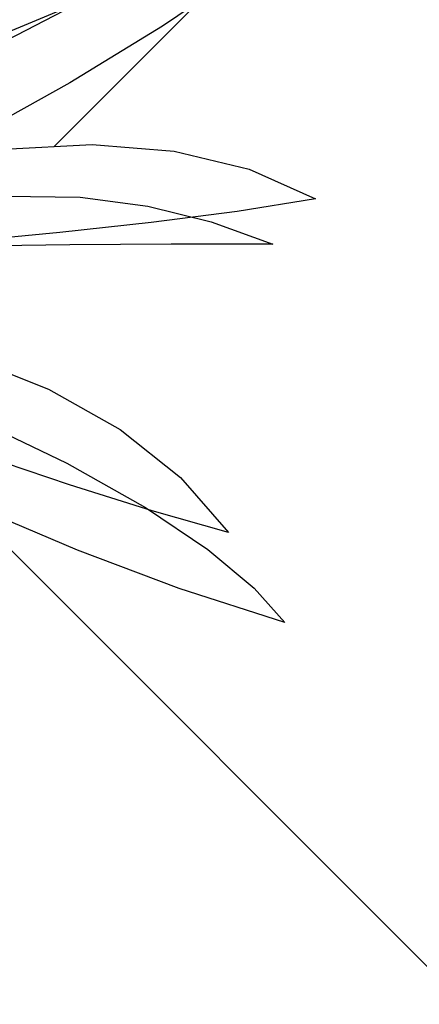
# Model space of a CAD drawing. Units: inches. Extents: x 3590 to 5167, y 65 to 1917.
# Tile 32 of 100: x 4960.64 to 4967.82, y 1339.27 to 1356.94. Entities that reach past the tile are written whole.
import ezdxf

# ---------------------------------------------------------------- set-up
doc = ezdxf.new("R2010")
doc.units = ezdxf.units.IN
doc.layers.add('A-FLOR-PATT', color=8, linetype='Continuous', lineweight=13)
doc.layers.add('L-PLNT', color=94, linetype='Continuous', lineweight=18)
doc.layers.add('DIENHOA', color=3, linetype='Continuous')

# ---------------------------------------------------------------- blocks, each defined once
blk = doc.blocks.new('Cay03_mb')
at = {"layer": 'DIENHOA'}
for p, q in [((363.69, 192.89), (290.19, 154.87)), ((314.63, 54.14), (369.18, 53.28)), ((369.18, 53.28), (418.6, 46.82)), ((418.6, 46.82), (464.87, 35.24)), ((464.87, 35.24), (510, 19)), ((361.61, 18.5), (289.03, 17.44)), ((435.8, 18.92), (361.61, 18.5)), ((510, 19), (435.8, 18.92)), ((289.55, -107.64), (359.29, -141.1)), ((359.29, -141.1), (416.89, -173.51)), ((367.1, -204.83), (296, -174.69)), ((416.89, -173.51), (462.55, -204.2)), ((441.55, -232.67), (367.1, -204.83)), ((462.55, -204.2), (496.5, -232.48)), ((518.93, -257.68), (441.55, -232.67)), ((496.5, -232.48), (518.93, -257.68))]:
    blk.add_line(p, q, dxfattribs=at)
for points in [[(496.74, 224.01), (429.38, 178.44), (361.6, 136.93), (294.07, 99.46), (227.46, 66.07), (162.44, 36.74), (99.68, 11.49), (39.84, -9.67), (-16.39, -26.73)], [(-16.39, -26.73), (75.38, 37.88), (160.06, 91.82), (237.27, 135.67), (306.57, 170.01), (367.58, 195.44), (419.88, 212.52), (463.07, 221.85), (496.74, 224.01)], [(23.69, -5.44), (99.27, 29.67), (173.22, 57.09), (244.79, 76.69), (313.26, 88.31), (377.88, 91.81), (437.93, 87.02), (492.67, 73.8), (541.37, 52)], [(541.37, 52), (484.11, 42.89), (421.18, 34.83), (354.36, 27.58), (285.41, 20.89), (216.1, 14.49), (148.2, 8.14), (83.47, 1.58), (23.69, -5.44)], [(-16.39, -26.73), (66.95, -26.58), (145.58, -32.71), (218.77, -44.94), (285.79, -63.12), (345.92, -87.06), (398.42, -116.6), (442.57, -151.57), (477.63, -191.79)], [(477.63, -191.79), (421.82, -176.03), (361.32, -156.94), (297.62, -135.49), (232.22, -112.64), (166.63, -89.37), (102.33, -66.65), (40.82, -45.45), (-16.39, -26.73)]]:
    blk.add_lwpolyline(points, dxfattribs=at)

msp = doc.modelspace()

# ---------------------------------------------------------------- hatches: boundary and pattern name
at = {"layer": 'A-FLOR-PATT', "transparency": 33554687}
h = msp.add_hatch(dxfattribs=at)
h.set_pattern_fill('AR-HBONE', color=256, scale=0.2)
h.set_pattern_definition([(45, (-588.972, 0), (0, 28.73682), [60.96, -20.32]), (135, (-574.604, 14.368), (3e-15, 28.73682), [60.96, -20.32])])
h.paths.add_polyline_path([(5071.274, 1796.999), (4933.274, 1796.999), (4933.274, 1753.999), (4962.774, 1753.999, -0.414214), (4928.774, 1719.999), (4933.274, 1718.999), (4933.274, 1334.999), (5071.274, 1334.999)])
h.paths.add_polyline_path([(4951.78, 1521.077), (4951.715, 1521.04), (4951.563, 1520.895)], flags=16)
h.paths.add_polyline_path([(4952.267, 1521.376), (4952.198, 1521.371), (4952.198, 1521.356)], flags=0)
h.paths.add_polyline_path([(4967.051, 1529.728), (4965.231, 1528.694), (4963.411, 1527.714), (4961.756, 1526.851), (4963.589, 1527.449), (4964.036, 1527.478), (4962.975, 1527.249), (4961.76, 1526.852), (4959.792, 1525.834), (4958.005, 1524.895), (4956.24, 1523.93), (4954.504, 1522.919), (4954.129, 1522.682), (4953.361, 1521.997), (4953.366, 1521.998), (4953.605, 1522.064), (4955.106, 1522.761), (4956.921, 1523.434), (4958.678, 1523.915), (4960.358, 1524.2), (4961.945, 1524.286), (4964.171, 1524.108), (4965.958, 1523.309), (4963.863, 1522.976), (4965.187, 1522.499), (4963.366, 1522.497), (4961.545, 1522.487), (4959.764, 1522.461), (4958.304, 1522.419), (4957.974, 1522.388), (4956.307, 1522.232), (4954.718, 1522.071), (4953.251, 1521.899), (4953.525, 1521.623), (4954.331, 1521.379), (4956.243, 1521.23), (4958.039, 1520.93), (4959.684, 1520.483), (4961.16, 1519.896), (4963.107, 1518.8), (4964.393, 1517.325), (4962.973, 1517.726), (4964.558, 1516.661), (4965.407, 1515.708), (4963.507, 1516.322), (4961.68, 1517.005), (4959.935, 1517.745), (4958.282, 1518.528), (4956.732, 1519.343), (4955.295, 1520.175), (4954.672, 1520.572), (4954.513, 1520.627), (4955.658, 1519.318), (4956.703, 1517.982), (4957.644, 1516.647), (4958.485, 1515.334), (4959.55, 1513.524), (4960.438, 1511.769), (4958.841, 1513.62), (4957.452, 1515.325), (4955.819, 1517.459), (4956.665, 1515.448), (4957.111, 1513.923), (4957.447, 1511.714), (4957.076, 1509.793), (4956.538, 1511.11), (4955.992, 1512.569), (4955.444, 1514.125), (4954.898, 1515.735), (4954.357, 1517.356), (4953.824, 1518.943), (4953.305, 1520.452), (4953.065, 1521.116), (4952.971, 1521.146), (4952.949, 1521.086), (4952.73, 1520.199), (4953.37, 1518.024), (4953.757, 1516.373), (4954.051, 1514.765), (4954.264, 1513.221), (4954.471, 1511.131), (4954.497, 1510.402), (4954.409, 1511.76), (4954.264, 1513.221), (4954.051, 1514.765), (4953.757, 1516.373), (4953.37, 1518.024), (4952.877, 1519.698), (4952.716, 1520.141), (4952.533, 1519.059), (4952.374, 1517.789), (4952.219, 1516.312), (4952.046, 1514.6), (4951.833, 1512.626), (4951.557, 1510.363), (4951.203, 1512.168), (4950.852, 1514.339), (4950.985, 1516.376), (4951.66, 1518.286), (4952.593, 1520.481), (4952.357, 1521.13), (4951.855, 1520.328), (4950.839, 1518.908), (4949.777, 1517.587), (4948.916, 1516.617), (4948.111, 1515.256), (4947.089, 1513.554), (4945.889, 1511.615), (4946.326, 1513.402), (4946.562, 1514.249), (4945.528, 1513.327), (4944.581, 1512.531), (4946.018, 1514.508), (4947.204, 1516.048), (4947.893, 1517.313), (4949.307, 1518.764), (4950.414, 1519.767), (4950.451, 1519.806), (4952.267, 1521.376), (4951.645, 1521.493), (4950.404, 1521.18), (4948.044, 1520.359), (4946.119, 1519.452), (4944.572, 1518.475), (4943.35, 1517.443), (4941.997, 1515.92), (4941.661, 1515.275), (4942.813, 1516.99), (4944.572, 1518.475), (4946.119, 1519.452), (4948.044, 1520.359), (4950.404, 1521.18), (4951.645, 1521.493), (4949.647, 1521.868), (4948.6, 1521.756), (4947.126, 1521.57), (4945.42, 1521.348), (4943.45, 1521.105), (4941.183, 1520.856), (4942.86, 1521.613), (4943.873, 1522.03), (4942.952, 1521.909), (4941.41, 1521.485), (4939.543, 1520.67), (4938.968, 1520.226), (4940.733, 1521.299), (4942.952, 1521.909), (4943.702, 1522.008), (4945.894, 1522.7), (4947.565, 1522.714), (4948.921, 1522.566), (4951.131, 1522.183), (4950.971, 1522.297), (4948.129, 1523.006), (4946.035, 1523.707), (4944.232, 1524.521), (4942.707, 1525.461), (4941.444, 1526.537), (4940.43, 1527.761), (4939.649, 1529.143), (4941.421, 1528.122), (4943.147, 1527.132), (4944.841, 1526.175), (4946.514, 1525.25), (4948.179, 1524.359), (4948.365, 1524.263), (4946.475, 1526.045), (4945.181, 1527.54), (4944.19, 1529.033), (4943.496, 1530.54), (4943.278, 1531.36), (4942.498, 1531.919), (4943.114, 1531.762), (4942.959, 1533.659), (4944.14, 1531.989), (4944.612, 1531.323), (4946.202, 1530.463), (4947.486, 1529.509), (4948.79, 1528.226), (4950.368, 1526.237), (4949.485, 1528.155), (4948.851, 1530.123), (4948.491, 1532.041), (4948.381, 1533.918), (4948.501, 1535.76), (4948.827, 1537.573), (4949.418, 1535.565), (4949.957, 1533.569), (4950.464, 1531.586), (4950.961, 1529.617), (4951.391, 1527.954), (4951.724, 1530.687), (4952.201, 1532.58), (4952.889, 1534.33), (4953.77, 1535.951), (4954.827, 1537.46), (4954.521, 1535.39), (4954.273, 1533.937), (4955.58, 1535.663), (4956.748, 1536.739), (4956.159, 1534.78), (4955.589, 1532.873), (4955.043, 1531.006), (4954.525, 1529.166), (4954.038, 1527.341), (4953.638, 1525.733), (4953.611, 1525.586), (4953.398, 1524.166), (4953.382, 1524.009), (4954.07, 1525.476), (4954.912, 1527.022), (4956.136, 1528.894), (4957.847, 1530.577), (4959.376, 1531.54), (4958.256, 1530.104), (4957.143, 1528.663), (4956.066, 1527.243), (4955.056, 1525.871), (4954.141, 1524.571), (4953.352, 1523.372), (4953.311, 1523.303), (4953.273, 1522.925), (4953.261, 1522.382), (4954.103, 1523.373), (4954.63, 1524.284), (4955.961, 1526.358), (4957.23, 1528.13), (4958.421, 1529.609), (4960.037, 1531.368), (4961.374, 1532.375), (4962.101, 1532.77), (4961.07, 1531.061), (4959.987, 1529.438), (4958.869, 1527.908), (4958.15, 1527.007), (4959.803, 1528.003), (4961.589, 1528.793), (4963.391, 1529.328), (4965.211, 1529.632)], flags=16)
h.paths.add_polyline_path([(4962.944, 1523.182), (4961.107, 1523.422), (4960.392, 1523.362), (4962.35, 1523.331)], flags=0)
h.paths.add_polyline_path([(5049.541, 1584.551), (5049.476, 1584.515), (5049.325, 1584.37)], flags=16)
h.paths.add_polyline_path([(5050.028, 1584.851), (5049.959, 1584.845), (5049.959, 1584.83)], flags=0)
h.paths.add_polyline_path([(5042.333, 1581.949), (5043.88, 1582.926), (5045.806, 1583.833), (5048.165, 1584.654), (5049.406, 1584.967), (5047.408, 1585.342), (5046.361, 1585.231), (5044.888, 1585.044), (5043.181, 1584.822), (5041.211, 1584.579), (5038.944, 1584.33), (5040.622, 1585.087), (5041.634, 1585.504), (5040.713, 1585.383), (5039.171, 1584.959), (5037.304, 1584.144), (5036.729, 1583.7), (5038.494, 1584.773), (5040.713, 1585.383), (5041.463, 1585.482), (5043.655, 1586.174), (5045.326, 1586.188), (5046.682, 1586.04), (5048.893, 1585.657), (5048.732, 1585.771), (5045.891, 1586.48), (5043.796, 1587.181), (5041.994, 1587.996), (5040.468, 1588.935), (5039.205, 1590.011), (5038.191, 1591.235), (5037.41, 1592.617), (5039.182, 1591.596), (5040.909, 1590.607), (5042.602, 1589.649), (5044.275, 1588.724), (5045.94, 1587.833), (5046.126, 1587.738), (5044.237, 1589.519), (5042.942, 1591.015), (5041.952, 1592.508), (5041.257, 1594.014), (5041.039, 1594.834), (5040.26, 1595.393), (5040.875, 1595.237), (5040.721, 1597.133), (5041.901, 1595.463), (5042.373, 1594.798), (5043.963, 1593.938), (5045.247, 1592.983), (5046.552, 1591.701), (5048.129, 1589.712), (5047.247, 1591.63), (5046.613, 1593.597), (5046.252, 1595.515), (5046.142, 1597.392), (5046.262, 1599.234), (5046.588, 1601.047), (5047.179, 1599.039), (5047.718, 1597.043), (5048.225, 1595.06), (5048.722, 1593.091), (5049.152, 1591.429), (5049.485, 1594.161), (5049.962, 1596.054), (5050.65, 1597.804), (5051.532, 1599.425), (5052.589, 1600.934), (5052.283, 1598.864), (5052.034, 1597.411), (5053.341, 1599.137), (5054.509, 1600.213), (5053.92, 1598.254), (5053.35, 1596.348), (5052.805, 1594.48), (5052.286, 1592.64), (5051.799, 1590.815), (5051.4, 1589.207), (5051.373, 1589.06), (5051.159, 1587.64), (5051.143, 1587.483), (5051.831, 1588.95), (5052.673, 1590.496), (5053.898, 1592.368), (5055.608, 1594.051), (5057.137, 1595.014), (5056.017, 1593.578), (5054.904, 1592.137), (5053.828, 1590.717), (5052.817, 1589.345), (5051.902, 1588.046), (5051.113, 1586.846), (5051.072, 1586.777), (5051.034, 1586.399), (5051.022, 1585.856), (5051.864, 1586.847), (5052.391, 1587.758), (5053.723, 1589.832), (5054.991, 1591.604), (5056.182, 1593.083), (5057.798, 1594.842), (5059.135, 1595.849), (5059.863, 1596.244), (5058.831, 1594.535), (5057.749, 1592.912), (5056.63, 1591.382), (5055.912, 1590.482), (5057.564, 1591.477), (5059.35, 1592.267), (5061.152, 1592.802), (5062.972, 1593.106), (5064.812, 1593.203), (5062.992, 1592.169), (5061.172, 1591.188), (5059.518, 1590.325), (5061.35, 1590.924), (5061.797, 1590.952), (5060.737, 1590.723), (5059.521, 1590.326), (5057.553, 1589.308), (5055.766, 1588.369), (5054.002, 1587.404), (5052.265, 1586.393), (5051.891, 1586.156), (5051.122, 1585.471), (5051.127, 1585.472), (5051.366, 1585.538), (5052.867, 1586.235), (5054.682, 1586.908), (5056.439, 1587.389), (5058.12, 1587.675), (5059.706, 1587.76), (5061.933, 1587.583), (5063.719, 1586.783), (5061.624, 1586.45), (5062.949, 1585.973), (5061.127, 1585.971), (5059.307, 1585.961), (5057.525, 1585.935), (5056.065, 1585.893), (5055.735, 1585.862), (5054.068, 1585.707), (5052.479, 1585.546), (5051.012, 1585.373), (5051.286, 1585.097), (5052.092, 1584.853), (5054.004, 1584.704), (5055.8, 1584.404), (5057.446, 1583.958), (5058.921, 1583.37), (5060.868, 1582.274), (5062.154, 1580.799), (5060.734, 1581.2), (5062.32, 1580.135), (5063.168, 1579.182), (5061.269, 1579.796), (5059.441, 1580.479), (5057.696, 1581.219), (5056.043, 1582.003), (5054.493, 1582.817), (5053.057, 1583.649), (5052.433, 1584.047), (5052.274, 1584.101), (5053.42, 1582.793), (5054.464, 1581.457), (5055.405, 1580.121), (5056.247, 1578.809), (5057.311, 1576.998), (5058.199, 1575.244), (5056.602, 1577.094), (5055.213, 1578.799), (5053.58, 1580.933), (5054.427, 1578.922), (5054.872, 1577.397), (5055.208, 1575.189), (5054.838, 1573.267), (5054.299, 1574.584), (5053.754, 1576.043), (5053.206, 1577.599), (5052.659, 1579.209), (5052.118, 1580.83), (5051.585, 1582.417), (5051.066, 1583.927), (5050.826, 1584.59), (5050.733, 1584.62), (5050.711, 1584.561), (5050.491, 1583.673), (5051.131, 1581.498), (5051.518, 1579.847), (5051.813, 1578.24), (5052.026, 1576.695), (5052.233, 1574.605), (5052.258, 1573.876), (5052.17, 1575.234), (5052.026, 1576.695), (5051.813, 1578.24), (5051.518, 1579.847), (5051.131, 1581.498), (5050.638, 1583.172), (5050.477, 1583.615), (5050.294, 1582.533), (5050.136, 1581.263), (5049.981, 1579.786), (5049.807, 1578.074), (5049.594, 1576.1), (5049.318, 1573.837), (5048.965, 1575.642), (5048.613, 1577.813), (5048.747, 1579.85), (5049.421, 1581.76), (5050.354, 1583.955), (5050.118, 1584.604), (5049.616, 1583.802), (5048.6, 1582.382), (5047.538, 1581.061), (5046.677, 1580.091), (5045.872, 1578.73), (5044.85, 1577.028), (5043.651, 1575.089), (5044.087, 1576.877), (5044.324, 1577.723), (5043.289, 1576.801), (5042.342, 1576.005), (5043.779, 1577.982), (5044.966, 1579.522), (5045.655, 1580.787), (5047.068, 1582.239), (5048.175, 1583.241), (5048.213, 1583.28), (5050.028, 1584.851), (5049.406, 1584.967), (5048.165, 1584.654), (5045.806, 1583.833), (5043.88, 1582.926), (5042.333, 1581.949), (5041.111, 1580.917), (5039.758, 1579.394), (5039.423, 1578.749), (5040.575, 1580.464)], flags=16)
h.paths.add_polyline_path([(4954.799, 1533.12), (4954.262, 1532.079), (4953.831, 1530.935), (4953.505, 1529.636), (4953.283, 1528.133), (4953.167, 1526.376), (4953.156, 1524.315), (4953.277, 1521.236), (4952.802, 1521.842), (4951.557, 1521.998), (4950.976, 1521.961), (4952.661, 1521.941), (4952.802, 1521.842), (4953.152, 1523.593), (4953.167, 1526.376), (4953.283, 1528.133), (4953.609, 1530.346), (4954.456, 1532.592)], flags=0)
h.paths.add_polyline_path([(5050.563, 1585.316), (5049.318, 1585.472), (5048.737, 1585.435), (5050.422, 1585.415), (5050.563, 1585.316), (5050.914, 1587.067), (5050.928, 1589.851), (5051.045, 1591.607), (5051.371, 1593.82), (5052.217, 1596.066), (5052.56, 1596.594), (5052.024, 1595.554), (5051.592, 1594.409), (5051.266, 1593.11), (5051.045, 1591.607), (5050.928, 1589.851), (5050.918, 1587.789), (5051.038, 1584.71)], flags=0)
h.paths.add_polyline_path([(5058.153, 1586.836), (5060.111, 1586.805), (5060.705, 1586.656), (5058.868, 1586.896)], flags=0)
h.paths.add_polyline_path([(5049.541, 1430.936), (5049.476, 1430.9), (5049.325, 1430.755)], flags=16)
h.paths.add_polyline_path([(5050.028, 1431.236), (5049.959, 1431.231), (5049.959, 1431.215)], flags=0)
h.paths.add_polyline_path([(5046.588, 1447.432), (5047.179, 1445.425), (5047.718, 1443.429), (5048.225, 1441.446), (5048.722, 1439.476), (5049.152, 1437.814), (5049.485, 1440.546), (5049.962, 1442.439), (5050.65, 1444.189), (5051.532, 1445.811), (5052.589, 1447.319), (5052.283, 1445.249), (5052.034, 1443.796), (5053.341, 1445.522), (5054.509, 1446.598), (5053.92, 1444.64), (5053.35, 1442.733), (5052.805, 1440.865), (5052.286, 1439.025), (5051.799, 1437.201), (5051.4, 1435.592), (5051.373, 1435.445), (5051.159, 1434.025), (5051.143, 1433.868), (5051.831, 1435.335), (5052.673, 1436.881), (5053.898, 1438.753), (5055.608, 1440.436), (5057.137, 1441.4), (5056.017, 1439.963), (5054.904, 1438.522), (5053.828, 1437.102), (5052.817, 1435.73), (5051.902, 1434.431), (5051.113, 1433.231), (5051.072, 1433.162), (5051.034, 1432.784), (5051.022, 1432.242), (5051.864, 1433.232), (5052.391, 1434.143), (5053.723, 1436.217), (5054.991, 1437.989), (5056.182, 1439.468), (5057.798, 1441.227), (5059.135, 1442.235), (5059.863, 1442.629), (5058.831, 1440.921), (5057.749, 1439.298), (5056.63, 1437.767), (5055.912, 1436.867), (5057.564, 1437.863), (5059.35, 1438.652), (5061.152, 1439.187), (5062.972, 1439.491), (5064.812, 1439.588), (5062.992, 1438.554), (5061.172, 1437.573), (5059.518, 1436.71), (5061.35, 1437.309), (5061.797, 1437.337), (5060.737, 1437.108), (5059.521, 1436.711), (5057.553, 1435.693), (5055.766, 1434.754), (5054.002, 1433.789), (5052.265, 1432.778), (5051.891, 1432.541), (5051.122, 1431.856), (5051.127, 1431.857), (5051.366, 1431.923), (5052.867, 1432.62), (5054.682, 1433.293), (5056.439, 1433.775), (5058.12, 1434.06), (5059.706, 1434.145), (5061.933, 1433.968), (5063.719, 1433.168), (5061.624, 1432.835), (5062.949, 1432.358), (5061.127, 1432.357), (5059.307, 1432.346), (5057.525, 1432.32), (5056.065, 1432.278), (5055.735, 1432.248), (5054.068, 1432.092), (5052.479, 1431.931), (5051.012, 1431.759), (5051.286, 1431.482), (5052.092, 1431.238), (5054.004, 1431.089), (5055.8, 1430.789), (5057.446, 1430.343), (5058.921, 1429.755), (5060.868, 1428.66), (5062.154, 1427.185), (5060.734, 1427.585), (5062.32, 1426.52), (5063.168, 1425.567), (5061.269, 1426.181), (5059.441, 1426.865), (5057.696, 1427.604), (5056.043, 1428.388), (5054.493, 1429.202), (5053.057, 1430.034), (5052.433, 1430.432), (5052.274, 1430.487), (5053.42, 1429.178), (5054.464, 1427.842), (5055.405, 1426.506), (5056.247, 1425.194), (5057.311, 1423.383), (5058.199, 1421.629), (5056.602, 1423.479), (5055.213, 1425.184), (5053.58, 1427.318), (5054.427, 1425.307), (5054.872, 1423.782), (5055.208, 1421.574), (5054.838, 1419.652), (5054.299, 1420.97), (5053.754, 1422.428), (5053.206, 1423.984), (5052.659, 1425.595), (5052.118, 1427.215), (5051.585, 1428.802), (5051.066, 1430.312), (5050.826, 1430.975), (5050.733, 1431.005), (5050.711, 1430.946), (5050.491, 1430.058), (5051.131, 1427.883), (5051.518, 1426.232), (5051.813, 1424.625), (5052.026, 1423.081), (5052.233, 1420.991), (5052.258, 1420.261), (5052.17, 1421.619), (5052.026, 1423.081), (5051.813, 1424.625), (5051.518, 1426.232), (5051.131, 1427.883), (5050.638, 1429.558), (5050.477, 1430.001), (5050.294, 1428.918), (5050.136, 1427.648), (5049.981, 1426.171), (5049.807, 1424.459), (5049.594, 1422.485), (5049.318, 1420.222), (5048.965, 1422.028), (5048.613, 1424.199), (5048.747, 1426.235), (5049.421, 1428.146), (5050.354, 1430.34), (5050.118, 1430.989), (5049.616, 1430.187), (5048.6, 1428.768), (5047.538, 1427.446), (5046.677, 1426.477), (5045.872, 1425.116), (5044.85, 1423.413), (5043.651, 1421.474), (5044.087, 1423.262), (5044.324, 1424.109), (5043.289, 1423.186), (5042.342, 1422.391), (5043.779, 1424.368), (5044.966, 1425.907), (5045.655, 1427.173), (5047.068, 1428.624), (5048.175, 1429.627), (5048.213, 1429.666), (5050.028, 1431.236), (5049.406, 1431.353), (5048.165, 1431.039), (5045.806, 1430.218), (5043.88, 1429.311), (5042.333, 1428.334), (5041.111, 1427.302), (5039.758, 1425.779), (5039.423, 1425.134), (5040.575, 1426.849), (5042.333, 1428.334), (5043.88, 1429.311), (5045.806, 1430.218), (5048.165, 1431.039), (5049.406, 1431.353), (5047.408, 1431.727), (5046.361, 1431.616), (5044.888, 1431.429), (5043.181, 1431.207), (5041.211, 1430.964), (5038.944, 1430.715), (5040.622, 1431.472), (5041.634, 1431.89), (5040.713, 1431.769), (5039.171, 1431.345), (5037.304, 1430.53), (5036.729, 1430.085), (5038.494, 1431.158), (5040.713, 1431.769), (5041.463, 1431.867), (5043.655, 1432.559), (5045.326, 1432.573), (5046.682, 1432.425), (5048.893, 1432.042), (5048.732, 1432.156), (5045.891, 1432.865), (5043.796, 1433.566), (5041.994, 1434.381), (5040.468, 1435.321), (5039.205, 1436.396), (5038.191, 1437.62), (5037.41, 1439.002), (5039.182, 1437.982), (5040.909, 1436.992), (5042.602, 1436.034), (5044.275, 1435.109), (5045.94, 1434.218), (5046.126, 1434.123), (5044.237, 1435.904), (5042.942, 1437.4), (5041.952, 1438.893), (5041.257, 1440.399), (5041.039, 1441.219), (5040.26, 1441.778), (5040.875, 1441.622), (5040.721, 1443.518), (5041.901, 1441.848), (5042.373, 1441.183), (5043.963, 1440.323), (5045.247, 1439.369), (5046.552, 1438.086), (5048.129, 1436.097), (5047.247, 1438.015), (5046.613, 1439.982), (5046.252, 1441.901), (5046.142, 1443.778), (5046.262, 1445.619)], flags=16)
h.paths.add_polyline_path([(5052.382, 1444.255), (5051.623, 1442.78), (5052.024, 1441.939), (5052.56, 1442.98)], flags=0)
h.paths.add_polyline_path([(5050.563, 1431.701), (5049.318, 1431.857), (5048.737, 1431.821), (5050.422, 1431.8)], flags=0)
h.paths.add_polyline_path([(5058.153, 1433.221), (5060.111, 1433.19), (5060.705, 1433.041), (5058.868, 1433.281)], flags=0)
h.paths.add_polyline_path([(5049.541, 1352.285), (5049.476, 1352.249), (5049.325, 1352.104)], flags=16)
h.paths.add_polyline_path([(5050.028, 1352.585), (5049.959, 1352.58), (5049.959, 1352.564)], flags=0)
h.paths.add_polyline_path([(5046.588, 1368.781), (5047.179, 1366.774), (5047.718, 1364.778), (5048.225, 1362.795), (5048.722, 1360.825), (5049.152, 1359.163), (5049.485, 1361.896), (5049.962, 1363.789), (5050.65, 1365.538), (5051.532, 1367.16), (5052.589, 1368.669), (5052.283, 1366.598), (5052.034, 1365.145), (5053.341, 1366.871), (5054.509, 1367.947), (5053.92, 1365.989), (5053.35, 1364.082), (5052.805, 1362.214), (5052.286, 1360.374), (5051.799, 1358.55), (5051.4, 1356.942), (5051.373, 1356.794), (5051.159, 1355.374), (5051.143, 1355.218), (5051.831, 1356.684), (5052.673, 1358.23), (5053.898, 1360.102), (5055.608, 1361.786), (5057.137, 1362.749), (5056.017, 1361.313), (5054.904, 1359.872), (5053.828, 1358.452), (5052.817, 1357.079), (5051.902, 1355.78), (5051.113, 1354.581), (5051.072, 1354.512), (5051.034, 1354.133), (5051.022, 1353.591), (5051.864, 1354.581), (5052.391, 1355.492), (5053.723, 1357.566), (5054.991, 1359.338), (5056.182, 1360.817), (5057.798, 1362.577), (5059.135, 1363.584), (5059.863, 1363.979), (5058.831, 1362.27), (5057.749, 1360.647), (5056.63, 1359.117), (5055.912, 1358.216), (5057.564, 1359.212), (5059.35, 1360.001), (5061.152, 1360.536), (5062.972, 1360.841), (5064.812, 1360.937), (5062.992, 1359.903), (5061.172, 1358.923), (5059.518, 1358.059), (5061.35, 1358.658), (5061.797, 1358.687), (5060.737, 1358.458), (5059.521, 1358.061), (5057.553, 1357.043), (5055.766, 1356.103), (5054.002, 1355.138), (5052.265, 1354.127), (5051.891, 1353.89), (5051.122, 1353.206), (5051.127, 1353.206), (5051.366, 1353.272), (5052.867, 1353.969), (5054.682, 1354.643), (5056.439, 1355.124), (5058.12, 1355.409), (5059.706, 1355.495), (5061.933, 1355.317), (5063.719, 1354.518), (5061.624, 1354.184), (5062.949, 1353.708), (5061.127, 1353.706), (5059.307, 1353.695), (5057.525, 1353.669), (5056.065, 1353.627), (5055.735, 1353.597), (5054.068, 1353.441), (5052.479, 1353.28), (5051.012, 1353.108), (5051.286, 1352.831), (5052.092, 1352.587), (5054.004, 1352.439), (5055.8, 1352.138), (5057.446, 1351.692), (5058.921, 1351.104), (5060.868, 1350.009), (5062.154, 1348.534), (5060.734, 1348.935), (5062.32, 1347.869), (5063.168, 1346.916), (5061.269, 1347.53), (5059.441, 1348.214), (5057.696, 1348.954), (5056.043, 1349.737), (5054.493, 1350.551), (5053.057, 1351.383), (5052.433, 1351.781), (5052.274, 1351.836), (5053.42, 1350.527), (5054.464, 1349.191), (5055.405, 1347.855), (5056.247, 1346.543), (5057.311, 1344.733), (5058.199, 1342.978), (5056.602, 1344.828), (5055.213, 1346.534), (5053.58, 1348.667), (5054.427, 1346.656), (5054.872, 1345.132), (5055.208, 1342.923), (5054.838, 1341.002), (5054.299, 1342.319), (5053.754, 1343.778), (5053.206, 1345.334), (5052.659, 1346.944), (5052.118, 1348.564), (5051.585, 1350.151), (5051.066, 1351.661), (5050.826, 1352.324), (5050.733, 1352.355), (5050.711, 1352.295), (5050.491, 1351.408), (5051.131, 1349.232), (5051.518, 1347.581), (5051.813, 1345.974), (5052.026, 1344.43), (5052.233, 1342.34), (5052.258, 1341.61), (5052.17, 1342.969), (5052.026, 1344.43), (5051.813, 1345.974), (5051.518, 1347.581), (5051.131, 1349.232), (5050.638, 1350.907), (5050.477, 1351.35), (5050.294, 1350.267), (5050.136, 1348.997), (5049.981, 1347.52), (5049.807, 1345.809), (5049.594, 1343.835), (5049.318, 1341.571), (5048.965, 1343.377), (5048.613, 1345.548), (5048.747, 1347.585), (5049.421, 1349.495), (5050.354, 1351.689), (5050.118, 1352.339), (5049.616, 1351.536), (5048.6, 1350.117), (5047.538, 1348.795), (5046.677, 1347.826), (5045.872, 1346.465), (5044.85, 1344.763), (5043.651, 1342.824), (5044.087, 1344.611), (5044.324, 1345.458), (5043.289, 1344.535), (5042.342, 1343.74), (5043.779, 1345.717), (5044.966, 1347.256), (5045.655, 1348.522), (5047.068, 1349.973), (5048.175, 1350.976), (5048.213, 1351.015), (5050.028, 1352.585), (5049.406, 1352.702), (5048.165, 1352.388), (5045.806, 1351.567), (5043.88, 1350.661), (5042.333, 1349.683), (5041.111, 1348.651), (5039.758, 1347.128), (5039.423, 1346.483), (5040.575, 1348.198), (5042.333, 1349.683), (5043.88, 1350.661), (5045.806, 1351.567), (5048.165, 1352.388), (5049.406, 1352.702), (5047.408, 1353.076), (5046.361, 1352.965), (5044.888, 1352.779), (5043.181, 1352.556), (5041.211, 1352.313), (5038.944, 1352.065), (5040.622, 1352.821), (5041.634, 1353.239), (5040.713, 1353.118), (5039.171, 1352.694), (5037.304, 1351.879), (5036.729, 1351.434), (5038.494, 1352.508), (5040.713, 1353.118), (5041.463, 1353.216), (5043.655, 1353.909), (5045.326, 1353.923), (5046.682, 1353.774), (5048.893, 1353.391), (5048.732, 1353.506), (5045.891, 1354.214), (5043.796, 1354.915), (5041.994, 1355.73), (5040.468, 1356.67), (5039.205, 1357.746), (5038.191, 1358.969), (5037.41, 1360.352), (5039.182, 1359.331), (5040.909, 1358.341), (5042.602, 1357.383), (5044.275, 1356.458), (5045.94, 1355.567), (5046.126, 1355.472), (5044.237, 1357.253), (5042.942, 1358.749), (5041.952, 1360.242), (5041.257, 1361.748), (5041.039, 1362.568), (5040.26, 1363.128), (5040.875, 1362.971), (5040.721, 1364.867), (5041.901, 1363.197), (5042.373, 1362.532), (5043.963, 1361.672), (5045.247, 1360.718), (5046.552, 1359.435), (5048.129, 1357.446), (5047.247, 1359.364), (5046.613, 1361.331), (5046.252, 1363.25), (5046.142, 1365.127), (5046.262, 1366.969)], flags=16)
h.paths.add_polyline_path([(5052.382, 1365.604), (5051.623, 1364.129), (5052.024, 1363.288), (5052.56, 1364.329)], flags=0)
h.paths.add_polyline_path([(4951.78, 1698.041), (4951.715, 1698.005), (4951.563, 1697.859)], flags=16)
h.paths.add_polyline_path([(4952.267, 1698.341), (4952.198, 1698.335), (4952.198, 1698.32)], flags=0)
h.paths.add_polyline_path([(4957.076, 1686.757), (4956.538, 1688.074), (4955.992, 1689.533), (4955.444, 1691.089), (4954.898, 1692.699), (4954.357, 1694.32), (4953.824, 1695.907), (4953.305, 1697.417), (4953.065, 1698.08), (4952.971, 1698.11), (4952.949, 1698.051), (4952.73, 1697.163), (4953.37, 1694.988), (4953.757, 1693.337), (4954.051, 1691.729), (4954.264, 1690.185), (4954.471, 1688.095), (4954.497, 1687.366), (4954.409, 1688.724), (4954.264, 1690.185), (4954.051, 1691.729), (4953.757, 1693.337), (4953.37, 1694.988), (4952.877, 1696.662), (4952.716, 1697.105), (4952.533, 1696.023), (4952.374, 1694.753), (4952.219, 1693.276), (4952.046, 1691.564), (4951.833, 1689.59), (4951.557, 1687.327), (4951.203, 1689.132), (4950.852, 1691.303), (4950.985, 1693.34), (4951.66, 1695.25), (4952.593, 1697.445), (4952.357, 1698.094), (4951.855, 1697.292), (4950.839, 1695.872), (4949.777, 1694.551), (4948.916, 1693.581), (4948.111, 1692.22), (4947.089, 1690.518), (4945.889, 1688.579), (4946.326, 1690.366), (4946.562, 1691.213), (4945.528, 1690.291), (4944.581, 1689.495), (4946.018, 1691.472), (4947.204, 1693.012), (4947.893, 1694.277), (4949.307, 1695.729), (4950.414, 1696.731), (4950.451, 1696.77), (4952.267, 1698.341), (4951.645, 1698.457), (4950.404, 1698.144), (4948.044, 1697.323), (4946.119, 1696.416), (4944.572, 1695.439), (4943.35, 1694.407), (4941.997, 1692.884), (4941.661, 1692.239), (4942.813, 1693.954), (4944.572, 1695.439), (4946.119, 1696.416), (4948.044, 1697.323), (4950.404, 1698.144), (4951.645, 1698.457), (4949.647, 1698.832), (4948.6, 1698.72), (4947.126, 1698.534), (4945.42, 1698.312), (4943.45, 1698.069), (4941.183, 1697.82), (4942.86, 1698.577), (4943.873, 1698.994), (4942.952, 1698.873), (4941.41, 1698.449), (4939.543, 1697.634), (4938.968, 1697.19), (4940.733, 1698.263), (4942.952, 1698.873), (4943.702, 1698.972), (4945.894, 1699.664), (4947.565, 1699.678), (4948.921, 1699.53), (4951.131, 1699.147), (4950.971, 1699.261), (4948.129, 1699.97), (4946.035, 1700.671), (4944.232, 1701.486), (4942.707, 1702.425), (4941.444, 1703.501), (4940.43, 1704.725), (4939.649, 1706.107), (4941.421, 1705.086), (4943.147, 1704.097), (4944.841, 1703.139), (4946.514, 1702.214), (4948.179, 1701.323), (4948.365, 1701.227), (4946.475, 1703.009), (4945.181, 1704.505), (4944.19, 1705.997), (4943.496, 1707.504), (4943.278, 1708.324), (4942.498, 1708.883), (4943.114, 1708.727), (4942.959, 1710.623), (4944.14, 1708.953), (4944.612, 1708.287), (4946.202, 1707.428), (4947.486, 1706.473), (4948.79, 1705.191), (4950.368, 1703.202), (4949.485, 1705.12), (4948.851, 1707.087), (4948.491, 1709.005), (4948.381, 1710.882), (4948.501, 1712.724), (4948.827, 1714.537), (4949.418, 1712.529), (4949.957, 1710.533), (4950.464, 1708.55), (4950.961, 1706.581), (4951.391, 1704.919), (4951.724, 1707.651), (4952.201, 1709.544), (4952.889, 1711.294), (4953.77, 1712.915), (4954.827, 1714.424), (4954.521, 1712.354), (4954.273, 1710.901), (4955.58, 1712.627), (4956.748, 1713.703), (4956.159, 1711.744), (4955.589, 1709.837), (4955.043, 1707.97), (4954.525, 1706.13), (4954.038, 1704.305), (4953.638, 1702.697), (4953.611, 1702.55), (4953.398, 1701.13), (4953.382, 1700.973), (4954.07, 1702.44), (4954.912, 1703.986), (4956.136, 1705.858), (4957.847, 1707.541), (4959.376, 1708.504), (4958.256, 1707.068), (4957.143, 1705.627), (4956.066, 1704.207), (4955.056, 1702.835), (4954.141, 1701.536), (4953.352, 1700.336), (4953.311, 1700.267), (4953.273, 1699.889), (4953.261, 1699.346), (4954.103, 1700.337), (4954.63, 1701.248), (4955.961, 1703.322), (4957.23, 1705.094), (4958.421, 1706.573), (4960.037, 1708.332), (4961.374, 1709.339), (4962.101, 1709.734), (4961.07, 1708.025), (4959.987, 1706.402), (4958.869, 1704.872), (4958.15, 1703.972), (4959.803, 1704.967), (4961.589, 1705.757), (4963.391, 1706.292), (4965.211, 1706.596), (4967.051, 1706.692), (4965.231, 1705.659), (4963.411, 1704.678), (4961.756, 1703.815), (4963.589, 1704.413), (4964.036, 1704.442), (4962.975, 1704.213), (4961.76, 1703.816), (4959.792, 1702.798), (4958.005, 1701.859), (4956.24, 1700.894), (4954.504, 1699.883), (4954.129, 1699.646), (4953.361, 1698.961), (4953.366, 1698.962), (4953.605, 1699.028), (4955.106, 1699.725), (4956.921, 1700.398), (4958.678, 1700.879), (4960.358, 1701.164), (4961.945, 1701.25), (4964.171, 1701.073), (4965.958, 1700.273), (4963.863, 1699.94), (4965.187, 1699.463), (4963.366, 1699.461), (4961.545, 1699.451), (4959.764, 1699.425), (4958.304, 1699.383), (4957.974, 1699.352), (4956.307, 1699.197), (4954.718, 1699.036), (4953.251, 1698.863), (4953.525, 1698.587), (4954.331, 1698.343), (4956.243, 1698.194), (4958.039, 1697.894), (4959.684, 1697.447), (4961.16, 1696.86), (4963.107, 1695.764), (4964.393, 1694.289), (4962.973, 1694.69), (4964.558, 1693.625), (4965.407, 1692.672), (4963.507, 1693.286), (4961.68, 1693.969), (4959.935, 1694.709), (4958.282, 1695.492), (4956.732, 1696.307), (4955.295, 1697.139), (4954.672, 1697.536), (4954.513, 1697.591), (4955.658, 1696.282), (4956.703, 1694.946), (4957.644, 1693.611), (4958.485, 1692.298), (4959.55, 1690.488), (4960.438, 1688.733), (4958.841, 1690.584), (4957.452, 1692.289), (4955.819, 1694.423), (4956.665, 1692.412), (4957.111, 1690.887), (4957.447, 1688.678)], flags=16)
h.paths.add_polyline_path([(5050.563, 1353.05), (5049.318, 1353.207), (5048.737, 1353.17), (5050.422, 1353.15)], flags=0)
h.paths.add_polyline_path([(4951.78, 1351.486), (4951.715, 1351.45), (4951.563, 1351.305)], flags=16)
h.paths.add_polyline_path([(4952.267, 1351.786), (4952.198, 1351.78), (4952.198, 1351.765)], flags=0)
h.paths.add_polyline_path([(4954.827, 1367.869), (4954.521, 1365.799), (4954.273, 1364.346), (4955.58, 1366.072), (4956.748, 1367.148), (4956.159, 1365.19), (4955.589, 1363.283), (4955.043, 1361.415), (4954.525, 1359.575), (4954.038, 1357.751), (4953.638, 1356.142), (4953.611, 1355.995), (4953.398, 1354.575), (4953.382, 1354.418), (4954.07, 1355.885), (4954.912, 1357.431), (4956.136, 1359.303), (4957.847, 1360.986), (4959.376, 1361.95), (4958.256, 1360.513), (4957.143, 1359.072), (4956.066, 1357.652), (4955.056, 1356.28), (4954.141, 1354.981), (4953.352, 1353.781), (4953.311, 1353.712), (4953.273, 1353.334), (4953.261, 1352.792), (4954.103, 1353.782), (4954.63, 1354.693), (4955.961, 1356.767), (4957.23, 1358.539), (4958.421, 1360.018), (4960.037, 1361.777), (4961.374, 1362.785), (4962.101, 1363.179), (4961.07, 1361.471), (4959.987, 1359.848), (4958.869, 1358.317), (4958.15, 1357.417), (4959.803, 1358.413), (4961.589, 1359.202), (4963.391, 1359.737), (4965.211, 1360.041), (4967.051, 1360.138), (4965.231, 1359.104), (4963.411, 1358.123), (4961.756, 1357.26), (4963.589, 1357.859), (4964.036, 1357.887), (4962.975, 1357.658), (4961.76, 1357.261), (4959.792, 1356.243), (4958.005, 1355.304), (4956.24, 1354.339), (4954.504, 1353.328), (4954.129, 1353.091), (4953.361, 1352.406), (4953.366, 1352.407), (4953.605, 1352.473), (4955.106, 1353.17), (4956.921, 1353.843), (4958.678, 1354.325), (4960.358, 1354.61), (4961.945, 1354.695), (4964.171, 1354.518), (4965.958, 1353.718), (4963.863, 1353.385), (4965.187, 1352.908), (4963.366, 1352.907), (4961.545, 1352.896), (4959.764, 1352.87), (4958.304, 1352.828), (4957.974, 1352.798), (4956.307, 1352.642), (4954.718, 1352.481), (4953.251, 1352.309), (4953.525, 1352.032), (4954.331, 1351.788), (4956.243, 1351.639), (4958.039, 1351.339), (4959.684, 1350.893), (4961.16, 1350.305), (4963.107, 1349.21), (4964.393, 1347.735), (4962.973, 1348.135), (4964.558, 1347.07), (4965.407, 1346.117), (4963.507, 1346.731), (4961.68, 1347.414), (4959.935, 1348.154), (4958.282, 1348.938), (4956.732, 1349.752), (4955.295, 1350.584), (4954.672, 1350.982), (4954.513, 1351.036), (4955.658, 1349.728), (4956.703, 1348.392), (4957.644, 1347.056), (4958.485, 1345.744), (4959.55, 1343.933), (4960.438, 1342.179), (4958.841, 1344.029), (4957.452, 1345.734), (4955.819, 1347.868), (4956.665, 1345.857), (4957.111, 1344.332), (4957.447, 1342.124), (4957.076, 1340.202), (4956.538, 1341.52), (4955.992, 1342.978), (4955.444, 1344.534), (4954.898, 1346.145), (4954.357, 1347.765), (4953.824, 1349.352), (4953.305, 1350.862), (4953.065, 1351.525), (4952.971, 1351.555), (4952.949, 1351.496), (4952.73, 1350.608), (4953.37, 1348.433), (4953.757, 1346.782), (4954.051, 1345.175), (4954.264, 1343.631), (4954.471, 1341.541), (4954.497, 1340.811), (4954.409, 1342.169), (4954.264, 1343.631), (4954.051, 1345.175), (4953.757, 1346.782), (4953.37, 1348.433), (4952.877, 1350.108), (4952.716, 1350.551), (4952.533, 1349.468), (4952.374, 1348.198), (4952.219, 1346.721), (4952.046, 1345.009), (4951.833, 1343.035), (4951.557, 1340.772), (4951.203, 1342.578), (4950.852, 1344.749), (4950.985, 1346.785), (4951.66, 1348.696), (4952.593, 1350.89), (4952.357, 1351.539), (4951.855, 1350.737), (4950.839, 1349.318), (4949.777, 1347.996), (4948.916, 1347.027), (4948.111, 1345.665), (4947.089, 1343.963), (4945.889, 1342.024), (4946.326, 1343.812), (4946.562, 1344.659), (4945.528, 1343.736), (4944.581, 1342.941), (4946.018, 1344.918), (4947.204, 1346.457), (4947.893, 1347.723), (4949.307, 1349.174), (4950.414, 1350.177), (4950.451, 1350.216), (4952.267, 1351.786), (4951.645, 1351.903), (4950.404, 1351.589), (4948.044, 1350.768), (4946.119, 1349.861), (4944.572, 1348.884), (4943.35, 1347.852), (4941.997, 1346.329), (4941.661, 1345.684), (4942.813, 1347.399), (4944.572, 1348.884), (4946.119, 1349.861), (4948.044, 1350.768), (4950.404, 1351.589), (4951.645, 1351.903), (4949.647, 1352.277), (4948.6, 1352.166), (4947.126, 1351.979), (4945.42, 1351.757), (4943.45, 1351.514), (4941.183, 1351.265), (4942.86, 1352.022), (4943.873, 1352.44), (4942.952, 1352.319), (4941.41, 1351.895), (4939.543, 1351.08), (4938.968, 1350.635), (4940.733, 1351.708), (4942.952, 1352.319), (4943.702, 1352.417), (4945.894, 1353.109), (4947.565, 1353.123), (4948.921, 1352.975), (4951.131, 1352.592), (4950.971, 1352.706), (4948.129, 1353.415), (4946.035, 1354.116), (4944.232, 1354.931), (4942.707, 1355.871), (4941.444, 1356.946), (4940.43, 1358.17), (4939.649, 1359.552), (4941.421, 1358.532), (4943.147, 1357.542), (4944.841, 1356.584), (4946.514, 1355.659), (4948.179, 1354.768), (4948.365, 1354.673), (4946.475, 1356.454), (4945.181, 1357.95), (4944.19, 1359.443), (4943.496, 1360.949), (4943.278, 1361.769), (4942.498, 1362.328), (4943.114, 1362.172), (4942.959, 1364.068), (4944.14, 1362.398), (4944.612, 1361.733), (4946.202, 1360.873), (4947.486, 1359.919), (4948.79, 1358.636), (4950.368, 1356.647), (4949.485, 1358.565), (4948.851, 1360.532), (4948.491, 1362.451), (4948.381, 1364.328), (4948.501, 1366.169), (4948.827, 1367.982), (4949.418, 1365.975), (4949.957, 1363.979), (4950.464, 1361.995), (4950.961, 1360.026), (4951.391, 1358.364), (4951.724, 1361.096), (4952.201, 1362.989), (4952.889, 1364.739), (4953.77, 1366.361)], flags=16)
h.paths.add_polyline_path([(4954.799, 1363.53), (4954.262, 1362.489), (4953.831, 1361.344), (4953.505, 1360.045), (4953.283, 1358.543), (4953.167, 1356.786), (4953.156, 1354.724), (4953.277, 1351.646), (4952.802, 1352.251), (4951.557, 1352.407), (4950.976, 1352.371), (4952.661, 1352.35), (4952.802, 1352.251), (4953.152, 1354.002), (4953.167, 1356.786), (4953.283, 1358.543), (4953.609, 1360.755), (4954.456, 1363.001)], flags=0)
h.paths.add_polyline_path([(4952.802, 1698.806), (4951.557, 1698.962), (4950.976, 1698.925), (4952.661, 1698.905), (4952.802, 1698.806), (4953.152, 1700.557), (4953.167, 1703.34), (4953.283, 1705.097), (4953.609, 1707.31), (4954.456, 1709.556), (4954.799, 1710.084), (4954.262, 1709.043), (4953.831, 1707.899), (4953.505, 1706.6), (4953.283, 1705.097), (4953.167, 1703.34), (4953.156, 1701.279), (4953.277, 1698.2)], flags=0)
h.paths.add_polyline_path([(4962.944, 1700.146), (4961.107, 1700.386), (4960.392, 1700.326), (4962.35, 1700.295)], flags=0)
h.paths.add_polyline_path([(5058.153, 1354.57), (5060.111, 1354.539), (5060.705, 1354.391), (5058.868, 1354.631)], flags=0)
h.paths.add_polyline_path([(4962.944, 1353.591), (4961.107, 1353.831), (4960.392, 1353.771), (4962.35, 1353.74)], flags=0)
h.paths.add_polyline_path([(5049.541, 1778.72), (5049.476, 1778.684), (5049.325, 1778.539)], flags=16)
h.paths.add_polyline_path([(5050.028, 1779.02), (5049.959, 1779.014), (5049.959, 1778.999)], flags=0)
h.paths.add_polyline_path([(5052.258, 1768.045), (5052.17, 1769.403), (5052.026, 1770.864), (5051.813, 1772.409), (5051.518, 1774.016), (5051.131, 1775.667), (5050.638, 1777.341), (5050.477, 1777.784), (5050.294, 1776.702), (5050.136, 1775.432), (5049.981, 1773.955), (5049.807, 1772.243), (5049.594, 1770.269), (5049.318, 1768.006), (5048.965, 1769.811), (5048.613, 1771.982), (5048.747, 1774.019), (5049.421, 1775.929), (5050.354, 1778.124), (5050.118, 1778.773), (5049.616, 1777.971), (5048.6, 1776.551), (5047.538, 1775.23), (5046.677, 1774.26), (5045.872, 1772.899), (5044.85, 1771.197), (5043.651, 1769.258), (5044.087, 1771.046), (5044.324, 1771.892), (5043.289, 1770.97), (5042.342, 1770.174), (5043.779, 1772.151), (5044.966, 1773.691), (5045.655, 1774.956), (5047.068, 1776.408), (5048.175, 1777.41), (5048.213, 1777.449), (5050.028, 1779.02), (5049.406, 1779.136), (5048.165, 1778.823), (5045.806, 1778.002), (5043.88, 1777.095), (5042.333, 1776.118), (5041.111, 1775.086), (5039.758, 1773.563), (5039.423, 1772.918), (5040.575, 1774.633), (5042.333, 1776.118), (5043.88, 1777.095), (5045.806, 1778.002), (5048.165, 1778.823), (5049.406, 1779.136), (5047.408, 1779.511), (5046.361, 1779.4), (5044.888, 1779.213), (5043.181, 1778.991), (5041.211, 1778.748), (5038.944, 1778.499), (5040.622, 1779.256), (5041.634, 1779.673), (5040.713, 1779.552), (5039.171, 1779.128), (5037.304, 1778.313), (5036.729, 1777.869), (5038.494, 1778.942), (5040.713, 1779.552), (5041.463, 1779.651), (5043.655, 1780.343), (5045.326, 1780.357), (5046.682, 1780.209), (5048.893, 1779.826), (5048.732, 1779.94), (5045.891, 1780.649), (5043.796, 1781.35), (5041.994, 1782.165), (5040.468, 1783.104), (5039.205, 1784.18), (5038.191, 1785.404), (5037.41, 1786.786), (5039.182, 1785.765), (5040.909, 1784.776), (5042.602, 1783.818), (5044.275, 1782.893), (5045.94, 1782.002), (5046.126, 1781.907), (5044.237, 1783.688), (5042.942, 1785.184), (5041.952, 1786.677), (5041.257, 1788.183), (5041.039, 1789.003), (5040.26, 1789.562), (5040.875, 1789.406), (5040.721, 1791.302), (5041.901, 1789.632), (5042.373, 1788.967), (5043.963, 1788.107), (5045.247, 1787.152), (5046.552, 1785.87), (5048.129, 1783.881), (5047.247, 1785.799), (5046.613, 1787.766), (5046.252, 1789.684), (5046.142, 1791.561), (5046.262, 1793.403), (5046.588, 1795.216), (5047.179, 1793.208), (5047.718, 1791.213), (5048.225, 1789.229), (5048.722, 1787.26), (5049.152, 1785.598), (5049.485, 1788.33), (5049.962, 1790.223), (5050.65, 1791.973), (5051.532, 1793.594), (5052.589, 1795.103), (5052.283, 1793.033), (5052.034, 1791.58), (5053.341, 1793.306), (5054.509, 1794.382), (5053.92, 1792.423), (5053.35, 1790.517), (5052.805, 1788.649), (5052.286, 1786.809), (5051.799, 1784.984), (5051.4, 1783.376), (5051.373, 1783.229), (5051.159, 1781.809), (5051.143, 1781.652), (5051.831, 1783.119), (5052.673, 1784.665), (5053.898, 1786.537), (5055.608, 1788.22), (5057.137, 1789.183), (5056.017, 1787.747), (5054.904, 1786.306), (5053.828, 1784.886), (5052.817, 1783.514), (5051.902, 1782.215), (5051.113, 1781.015), (5051.072, 1780.946), (5051.034, 1780.568), (5051.022, 1780.025), (5051.864, 1781.016), (5052.391, 1781.927), (5053.723, 1784.001), (5054.991, 1785.773), (5056.182, 1787.252), (5057.798, 1789.011), (5059.135, 1790.018), (5059.863, 1790.413), (5058.831, 1788.704), (5057.749, 1787.081), (5056.63, 1785.551), (5055.912, 1784.651), (5057.564, 1785.646), (5059.35, 1786.436), (5061.152, 1786.971), (5062.972, 1787.275), (5064.812, 1787.372), (5062.992, 1786.338), (5061.172, 1785.357), (5059.518, 1784.494), (5061.35, 1785.093), (5061.797, 1785.121), (5060.737, 1784.892), (5059.521, 1784.495), (5057.553, 1783.477), (5055.766, 1782.538), (5054.002, 1781.573), (5052.265, 1780.562), (5051.891, 1780.325), (5051.122, 1779.64), (5051.127, 1779.641), (5051.366, 1779.707), (5052.867, 1780.404), (5054.682, 1781.077), (5056.439, 1781.558), (5058.12, 1781.844), (5059.706, 1781.929), (5061.933, 1781.752), (5063.719, 1780.952), (5061.624, 1780.619), (5062.949, 1780.142), (5061.127, 1780.14), (5059.307, 1780.13), (5057.525, 1780.104), (5056.065, 1780.062), (5055.735, 1780.031), (5054.068, 1779.876), (5052.479, 1779.715), (5051.012, 1779.542), (5051.286, 1779.266), (5052.092, 1779.022), (5054.004, 1778.873), (5055.8, 1778.573), (5057.446, 1778.127), (5058.921, 1777.539), (5060.868, 1776.443), (5062.154, 1774.968), (5060.734, 1775.369), (5062.32, 1774.304), (5063.168, 1773.351), (5061.269, 1773.965), (5059.441, 1774.648), (5057.696, 1775.388), (5056.043, 1776.172), (5054.493, 1776.986), (5053.057, 1777.818), (5052.433, 1778.216), (5052.274, 1778.27), (5053.42, 1776.962), (5054.464, 1775.626), (5055.405, 1774.29), (5056.247, 1772.978), (5057.311, 1771.167), (5058.199, 1769.413), (5056.602, 1771.263), (5055.213, 1772.968), (5053.58, 1775.102), (5054.427, 1773.091), (5054.872, 1771.566), (5055.208, 1769.358), (5054.838, 1767.436), (5054.299, 1768.753), (5053.754, 1770.212), (5053.206, 1771.768), (5052.659, 1773.378), (5052.118, 1774.999), (5051.585, 1776.586), (5051.066, 1778.096), (5050.826, 1778.759), (5050.733, 1778.789), (5050.711, 1778.73), (5050.491, 1777.842), (5051.131, 1775.667), (5051.518, 1774.016), (5051.813, 1772.409), (5052.026, 1770.864), (5052.233, 1768.774)], flags=16)
h.paths.add_polyline_path([(5050.563, 1779.485), (5049.318, 1779.641), (5048.737, 1779.604), (5050.422, 1779.584), (5050.563, 1779.485), (5050.914, 1781.236), (5050.928, 1784.02), (5051.045, 1785.776), (5051.371, 1787.989), (5052.217, 1790.235), (5052.56, 1790.763), (5052.024, 1789.723), (5051.592, 1788.578), (5051.266, 1787.279), (5051.045, 1785.776), (5050.928, 1784.02), (5050.918, 1781.958), (5051.038, 1778.879)], flags=0)
h.paths.add_polyline_path([(5058.153, 1781.005), (5060.111, 1780.974), (5060.705, 1780.825), (5058.868, 1781.065)], flags=0)

# ---------------------------------------------------------------- block references
at = {"layer": 'L-PLNT', "xscale": 0.0245452446402784, "yscale": 0.0245452446402784, "zscale": 0.0245452446402784}
msp.add_blockref('Cay03_mb', (4952.669, 1352.442), dxfattribs=at)

doc.saveas('drawing.dxf')
